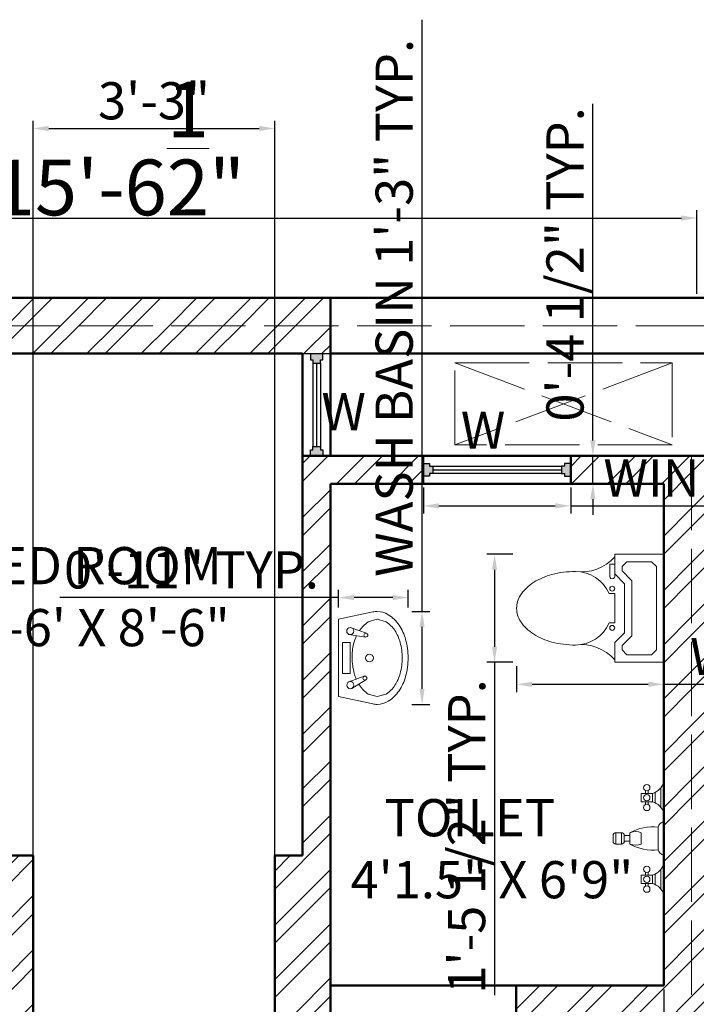
# Model space of a CAD drawing. Units: millimetres. Extents: x 4237 to 5109, y 21391 to 22486.
# Tile 9 of 17: x 4349 to 4458, y 22327 to 22486. Entities that reach past the tile are written whole.
import ezdxf

# ---------------------------------------------------------------- set-up
doc = ezdxf.new("R2010")
doc.units = ezdxf.units.MM
doc.linetypes.add('ACAD_ISO02W100', pattern=[15, 12, -3])
for name, color, linetype, lineweight in [('A-ANNO-DIMS', 2, 'Continuous', 18), ('A-ANNO-TEXT', 7, 'Continuous', 18), ('A-AREA-IDEN', 3, 'Continuous', 18), ('A-FLOR-OVHD', 1, 'ACAD_ISO02W100', 18), ('A-FURN', 8, 'Continuous', 18), ('A-WALL', 7, 'Continuous', 50), ('A-WALL-PATT', 252, 'Continuous', 13), ('windows', 140, 'Continuous', 25)]:
    doc.layers.add(name, color=color, linetype=linetype, lineweight=lineweight)
doc.styles.get("Standard").update_dxf_attribs({"font": 'arial.ttf'})
doc.dimstyles.new('ISO-25', dxfattribs={"dimtxt": 6, "dimasz": 2.5, "dimexe": 1.25, "dimexo": 0.625, "dimtad": 1, "dimdec": 1, "dimlunit": 4, "dimtxsty": 'Standard', "dimcen": 2.5, "dimadec": 0, "dimazin": 0, "dimtfac": 1, "dimtdec": 1, "dimtmove": 0, "dimatfit": 3, "dimfxl": 1, "dimarcsym": 0})

# ---------------------------------------------------------------- blocks, each defined once
blk = doc.blocks.new('A$C60F95712')
for p, q in [((0.05, 0.45), (0.003, 0.2283)), ((0.55, 0.45), (0.05, 0.45)), ((0.597, 0.2283), (0.55, 0.45)), ((0.1448, 0.3831), (0.1814, 0.2836)), ((0.4, 0.425), (0.2, 0.425)), ((0.2, 0.425), (0.2, 0.375)), ((0.4, 0.375), (0.4, 0.425)), ((0.1035, 0.3639), (0.1588, 0.2727)), ((0.2, 0.375), (0.4, 0.375)), ((0.4514, 0.3804), (0.4348, 0.2751)), ((0.4953, 0.3684), (0.459, 0.2688))]:
    blk.add_line(p, q)
for points in [[(0.1307, 0.319, 0.008163), (0.1232, 0.3143, 0.107176), (0.0669, 0.2578), (0.05, 0.2), (0.0669, 0.1422, 0.107176), (0.1232, 0.0857, 0.078233), (0.2003, 0.0515, 0.065516), (0.3, 0.0383, 0.065516), (0.3997, 0.0515, 0.078233), (0.4768, 0.0857, 0.107176), (0.5331, 0.1422), (0.55, 0.2)], [(0.4439, 0.3328, 0.046779), (0.3911, 0.3524, 0.080145), (0.3, 0.3617, 0.065516), (0.2003, 0.3485, 0.037125), (0.1623, 0.3353, 0.107176)], [(0.55, 0.2), (0.5331, 0.2578, 0.107176), (0.4768, 0.3143, 0.000976), (0.4758, 0.3149, 0.080145)]]:
    blk.add_lwpolyline(points, format="xyb")
for centre, radius in [((0.1241, 0.3735), 0.0228), ((0.4733, 0.3744), 0.0228), ((0.1696, 0.2793), 0.0126), ((0.3, 0.25), 0.025), ((0.4472, 0.2731), 0.0126)]:
    blk.add_circle(centre, radius)
for centre, radius, start, end in [((0.1362, 0.2), 0.1362, 168.02396, 180), ((0.1362, 0.2), 0.1362, 180, 211.85353), ((0.4638, 0.2), 0.1362, 328.14647, 0), ((0.4638, 0.2), 0.1362, 0, 11.97604), ((0.2147, 0.2488), 0.2286, 211.85353, 236.30993), ((0.3853, 0.2488), 0.2286, 303.69007, 328.14647), ((0.2662, 0.3261), 0.3215, 236.30993, 254.56292), ((0.3, 0.4484), 0.4484, 254.56292, 270), ((0.3, 0.4484), 0.4484, 270, 285.43708), ((0.3338, 0.3261), 0.3215, 285.43708, 303.69007)]:
    blk.add_arc(centre, radius, start, end)
blk = doc.blocks.new('A$C5EF6120A')
at = {"linetype": 'ByBlock'}
for p, q in [((0, 0.762), (0, 0.508)), ((0, 0.762), (0.5588, 0.762)), ((0.0381, 0.6985), (0.0635, 0.7239)), ((0.0635, 0.7239), (0.4953, 0.7239)), ((0.4953, 0.7239), (0.5207, 0.6985)), ((0.5588, 0.762), (0.5588, 0.508)), ((0.0381, 0.6985), (0.0381, 0.5715)), ((0.5207, 0.6985), (0.5207, 0.5715)), ((0.0635, 0.5461), (0.0381, 0.5715)), ((0.1366, 0.5969), (0.0858, 0.5461)), ((0.1366, 0.5969), (0.4222, 0.5969)), ((0.4222, 0.5969), (0.473, 0.5461)), ((0.5207, 0.5715), (0.4953, 0.5461)), ((0.0635, 0.5461), (0.0858, 0.5461)), ((0.1524, 0.5588), (0.1016, 0.508)), ((0.1524, 0.5588), (0.4064, 0.5588)), ((0.4064, 0.5588), (0.4572, 0.508)), ((0.4953, 0.5461), (0.473, 0.5461)), ((0, 0.508), (0.1016, 0.508)), ((0.0508, 0.508), (0.0508, 0.4826)), ((0.0508, 0.4826), (0.1143, 0.4826)), ((0.1143, 0.508), (0.1016, 0.508)), ((0.2032, 0.508), (0.2032, 0.4794)), ((0.3556, 0.508), (0.2032, 0.508)), ((0.3556, 0.508), (0.3556, 0.4794)), ((0.5588, 0.508), (0.4572, 0.508))]:
    blk.add_line(p, q, dxfattribs=at)
blk.add_lwpolyline([(0.0889, 0.3048, 0.063415), (0.1044, 0.183, 0.076468), (0.1447, 0.0893, 0.107136), (0.2118, 0.0204, 0.147373), (0.2794, 0, 0.147373), (0.347, 0.0204, 0.107136), (0.4141, 0.0893, 0.076468), (0.4544, 0.183, 0.063415), (0.4699, 0.3048, 0.063415)], format="xyb", dxfattribs=at)
for centre in [(0.1778, 0.4953), (0.381, 0.4953)]:
    blk.add_circle(centre, 0.0127, dxfattribs=at)
for centre, radius, start, end in [((-0.1375, 0.3358), 0.2285, 352.2011, 48.911), ((0.2794, 0.3048), 0.1905, 113.5782, 180), ((0.1143, 0.4953), 0.0127, 270, 90), ((0.2794, 0.3048), 0.1905, 0, 66.4218), ((0.6963, 0.3358), 0.2285, 131.089, 187.7989)]:
    blk.add_arc(centre, radius, start, end, dxfattribs=at)
blk = doc.blocks.new('Faucet - Bathroom front')
for p, q in [((-0.5, 4.25), (0.5, 4.25)), ((0.5, 3.75), (-0.5, 3.75)), ((-0.25, 3), (-0.25, 3.5)), ((0.25, 3.5), (0.25, 3)), ((-0.5, 3), (0.5, 3)), ((0.5, 2), (-0.5, 2)), ((-4, 1.625), (-4.25, 1.625)), ((-4, 1.375), (-4.25, 1.375)), ((-3.25, 1.625), (-3, 1.625)), ((-3.25, 1.375), (-3, 1.375)), ((3.25, 1.625), (3, 1.625)), ((3.25, 1.375), (3, 1.375)), ((4, 1.625), (4.25, 1.625)), ((4, 1.375), (4.25, 1.375)), ((-5, 0), (-2.25, 0)), ((-4.5087, 0.25), (-2.7408, 0.25)), ((-3.1442, 0.75), (-4.0979, 0.75)), ((-1.5, 0), (1.5, 0)), ((-1, 0.5), (1, 0.5)), ((2.25, 0), (5, 0)), ((2.7413, 0.25), (4.5092, 0.25)), ((4.1058, 0.75), (3.1521, 0.75))]:
    blk.add_line(p, q)
for points in [[(-0.25, 4.5), (0.25, 4.5)], [(-0.5, 3.75), (-0.5, 4.25)], [(0.25, 3.5), (-0.25, 3.5)], [(0.5, 4.25), (0.5, 3.75)]]:
    blk.add_lwpolyline(points)
for points in [[(-4, 1), (-4, 2), (-3.25, 2), (-3.25, 1)], [(3.25, 1), (3.25, 2), (4, 2), (4, 1)]]:
    blk.add_lwpolyline(points, close=True)
for centre in [(-4.5, 1.5), (-3.625, 1.5), (-2.75, 1.5), (2.75, 1.5), (3.625, 1.5), (4.5, 1.5)]:
    blk.add_circle(centre, 0.2795)
for centre, radius, start, end in [((-0.2575, 4.2575), 0.2426, 88.22243, 181.7776), ((0.2575, 4.2575), 0.2426, 358.2224, 91.77757), ((-0.2575, 3.7425), 0.2426, 178.2224, 271.7776), ((0.2575, 3.7425), 0.2426, 268.2224, 1.777565), ((3, 1), 4.0311, 150.2551, 187.125), ((0.6413, 2.5), 1.246, 156.3417, 203.6583), ((-3, 1), 4.0311, 352.875, 29.74488), ((-0.6413, 2.5), 1.246, 336.3417, 23.65835), ((-5.375, 1.375), 1.4252, 285.2551, 344.7449), ((-1.875, 1.375), 1.4252, 195.2551, 254.7449), ((1.875, 1.375), 1.4252, 285.2551, 344.7449), ((5.375, 1.375), 1.4252, 195.2551, 254.7449), ((-0.7962, -0.2038), 0.7327, 106.1502, 163.8498), ((0.7962, -0.2038), 0.7327, 16.1502, 73.84979)]:
    blk.add_arc(centre, radius, start, end)
blk = doc.blocks.new('*D56')
at = {"layer": 'A-ANNO-DIMS', "color": 0, "lineweight": -2, "transparency": 16777216}
for p, q in [((4271.65, 22441.33), (4271.65, 22454.84)), ((4458.3, 22441.33), (4458.3, 22454.84)), ((4274.15, 22453.59), (4455.8, 22453.59))]:
    blk.add_line(p, q, dxfattribs=at)
at = {"layer": 'A-ANNO-DIMS', "color": 0, "transparency": 16777216}
for points in [[(4274.15, 22454.01), (4274.15, 22453.17), (4271.65, 22453.59)], [(4455.8, 22454.01), (4455.8, 22453.17), (4458.3, 22453.59)]]:
    blk.add_solid(points, dxfattribs=at)
at = {"layer": 'Defpoints', "color": 0, "transparency": 16777216}
for p in [(4458.3, 22453.59), (4271.65, 22440.7), (4458.3, 22440.7)]:
    blk.add_point(p, dxfattribs=at)
at = {"layer": 'A-ANNO-DIMS', "color": 0, "transparency": 16777216, "insert": (4364.98, 22464.83), "char_height": 9, "attachment_point": 5}
blk.add_mtext('15\'-6{\\H1x;\\S1/2;}"', dxfattribs=at)
blk = doc.blocks.new('WIN-A')
blk.add_line((0, 4.5), (0, 0))
blk.add_lwpolyline([(0, 4.5), (23.8, 4.5), (23.8, 0), (0, 0)], close=True)
blk = doc.blocks.new('*D74')
at = {"layer": 'A-ANNO-DIMS', "color": 0, "lineweight": -2, "transparency": 16777216}
for p, q in [((4413.94, 22390.08), (4413.94, 22485.61)), ((4412.31, 22390.08), (4415.19, 22390.08)), ((4413.94, 22377.59), (4413.94, 22387.58)), ((4412.31, 22375.09), (4415.19, 22375.09))]:
    blk.add_line(p, q, dxfattribs=at)
at = {"layer": 'A-ANNO-DIMS', "color": 0, "transparency": 16777216}
for points in [[(4413.52, 22387.58), (4414.35, 22387.58), (4413.94, 22390.08)], [(4413.52, 22377.59), (4414.35, 22377.59), (4413.94, 22375.09)]]:
    blk.add_solid(points, dxfattribs=at)
at = {"layer": 'Defpoints', "color": 0, "transparency": 16777216}
for p in [(4411.69, 22390.08), (4413.94, 22390.08), (4411.69, 22375.09)]:
    blk.add_point(p, dxfattribs=at)
at = {"layer": 'A-ANNO-DIMS', "color": 0, "transparency": 16777216, "insert": (4410.21, 22439.09), "char_height": 6, "attachment_point": 5, "rotation": 90}
blk.add_mtext('WASH BASIN 1\'-3" TYP.', dxfattribs=at)
blk = doc.blocks.new('*D75')
at = {"layer": 'A-ANNO-DIMS', "color": 0, "lineweight": -2, "transparency": 16777216}
for p, q in [((4400.45, 22390.71), (4400.45, 22393.58)), ((4411.69, 22390.71), (4411.69, 22393.58)), ((4400.45, 22392.33), (4355.46, 22392.33)), ((4409.19, 22392.33), (4402.95, 22392.33))]:
    blk.add_line(p, q, dxfattribs=at)
at = {"layer": 'A-ANNO-DIMS', "color": 0, "transparency": 16777216}
for points in [[(4402.95, 22392.75), (4402.95, 22391.91), (4400.45, 22392.33)], [(4409.19, 22392.75), (4409.19, 22391.91), (4411.69, 22392.33)]]:
    blk.add_solid(points, dxfattribs=at)
at = {"layer": 'Defpoints', "color": 0, "transparency": 16777216}
for p in [(4400.45, 22392.33), (4400.45, 22390.08), (4411.69, 22390.08)]:
    blk.add_point(p, dxfattribs=at)
at = {"layer": 'A-ANNO-DIMS', "color": 0, "transparency": 16777216, "insert": (4376.7, 22396.02), "char_height": 6, "attachment_point": 5}
blk.add_mtext('0\'-11" TYP.', dxfattribs=at)
blk = doc.blocks.new('*D76')
at = {"layer": 'A-ANNO-DIMS', "color": 0, "lineweight": -2, "transparency": 16777216}
for p, q in [((4429.2, 22381.26), (4429.2, 22377.08)), ((4452.95, 22381.26), (4452.95, 22377.08)), ((4431.7, 22378.33), (4450.45, 22378.33)), ((4452.95, 22378.33), (4509.81, 22378.33))]:
    blk.add_line(p, q, dxfattribs=at)
at = {"layer": 'A-ANNO-DIMS', "color": 0, "transparency": 16777216}
for points in [[(4431.7, 22378.74), (4431.7, 22377.91), (4429.2, 22378.33)], [(4450.45, 22378.74), (4450.45, 22377.91), (4452.95, 22378.33)]]:
    blk.add_solid(points, dxfattribs=at)
at = {"layer": 'Defpoints', "color": 0, "transparency": 16777216}
for p in [(4429.2, 22381.89), (4452.95, 22381.89), (4452.95, 22378.33)]:
    blk.add_point(p, dxfattribs=at)
at = {"layer": 'A-ANNO-DIMS', "color": 0, "transparency": 16777216, "insert": (4482.63, 22382.05), "char_height": 6, "attachment_point": 5}
blk.add_mtext('WC 2\'-0" TYP.', dxfattribs=at)
blk = doc.blocks.new('*D77')
at = {"layer": 'A-ANNO-DIMS', "color": 0, "lineweight": -2, "transparency": 16777216}
for p, q in [((4428.57, 22399.31), (4424.39, 22399.31)), ((4425.64, 22396.81), (4425.64, 22384.39)), ((4428.57, 22381.89), (4424.39, 22381.89)), ((4425.64, 22381.89), (4425.64, 22328.15))]:
    blk.add_line(p, q, dxfattribs=at)
at = {"layer": 'A-ANNO-DIMS', "color": 0, "transparency": 16777216}
for points in [[(4425.22, 22396.81), (4426.05, 22396.81), (4425.64, 22399.31)], [(4425.22, 22384.39), (4426.05, 22384.39), (4425.64, 22381.89)]]:
    blk.add_solid(points, dxfattribs=at)
at = {"layer": 'Defpoints', "color": 0, "transparency": 16777216}
for p in [(4429.2, 22399.31), (4425.64, 22381.89), (4429.2, 22381.89)]:
    blk.add_point(p, dxfattribs=at)
at = {"layer": 'A-ANNO-DIMS', "color": 0, "transparency": 16777216, "insert": (4421.91, 22353.77), "char_height": 6, "attachment_point": 5, "rotation": 90}
blk.add_mtext('1\'-5 1/2" TYP.', dxfattribs=at)
blk = doc.blocks.new('*D80')
at = {"layer": 'A-ANNO-DIMS', "color": 0, "lineweight": -2, "transparency": 16777216}
for p, q in [((4414.15, 22410.08), (4414.15, 22405.88)), ((4437.95, 22410.08), (4437.95, 22405.88)), ((4416.65, 22407.13), (4435.45, 22407.13)), ((4437.95, 22407.13), (4527.87, 22407.13))]:
    blk.add_line(p, q, dxfattribs=at)
at = {"layer": 'A-ANNO-DIMS', "color": 0, "transparency": 16777216}
for points in [[(4416.65, 22407.55), (4416.65, 22406.71), (4414.15, 22407.13)], [(4435.45, 22407.55), (4435.45, 22406.71), (4437.95, 22407.13)]]:
    blk.add_solid(points, dxfattribs=at)
at = {"layer": 'Defpoints', "color": 0, "transparency": 16777216}
for p in [(4414.15, 22410.7), (4437.95, 22410.7), (4437.95, 22407.13)]:
    blk.add_point(p, dxfattribs=at)
at = {"layer": 'A-ANNO-DIMS', "color": 0, "transparency": 16777216, "insert": (4484.16, 22410.86), "char_height": 6, "attachment_point": 5}
blk.add_mtext('WINDOW W 2\'-0" TYP.', dxfattribs=at)
blk = doc.blocks.new('*D81')
at = {"layer": 'A-ANNO-DIMS', "color": 0, "lineweight": -2, "transparency": 16777216}
for p, q in [((4441.52, 22417.7), (4441.52, 22472)), ((4438.58, 22415.2), (4442.77, 22415.2)), ((4441.52, 22410.7), (4441.52, 22415.2)), ((4438.58, 22410.7), (4442.77, 22410.7)), ((4441.52, 22408.2), (4441.52, 22405.7))]:
    blk.add_line(p, q, dxfattribs=at)
at = {"layer": 'A-ANNO-DIMS', "color": 0, "transparency": 16777216}
for points in [[(4441.1, 22417.7), (4441.94, 22417.7), (4441.52, 22415.2)], [(4441.1, 22408.2), (4441.94, 22408.2), (4441.52, 22410.7)]]:
    blk.add_solid(points, dxfattribs=at)
at = {"layer": 'Defpoints', "color": 0, "transparency": 16777216}
for p in [(4437.95, 22415.2), (4441.52, 22415.2), (4437.95, 22410.7)]:
    blk.add_point(p, dxfattribs=at)
at = {"layer": 'A-ANNO-DIMS', "color": 0, "transparency": 16777216, "insert": (4437.79, 22446.1), "char_height": 6, "attachment_point": 5, "rotation": 90}
blk.add_mtext('0\'-4 1/2" TYP.', dxfattribs=at)
blk = doc.blocks.new('*D109')
at = {"layer": 'A-ANNO-DIMS', "color": 0, "lineweight": -2, "transparency": 16777216}
for p, q in [((4351.15, 22325.83), (4351.15, 22469.3)), ((4390.15, 22325.83), (4390.15, 22469.3)), ((4353.65, 22468.05), (4387.65, 22468.05))]:
    blk.add_line(p, q, dxfattribs=at)
at = {"layer": 'A-ANNO-DIMS', "color": 0, "transparency": 16777216}
for points in [[(4353.65, 22468.47), (4353.65, 22467.63), (4351.15, 22468.05)], [(4387.65, 22468.47), (4387.65, 22467.63), (4390.15, 22468.05)]]:
    blk.add_solid(points, dxfattribs=at)
at = {"layer": 'Defpoints', "color": 0, "transparency": 16777216}
for p in [(4390.15, 22468.05), (4351.15, 22325.2), (4390.15, 22325.2)]:
    blk.add_point(p, dxfattribs=at)
at = {"layer": 'A-ANNO-DIMS', "color": 0, "transparency": 16777216, "insert": (4370.65, 22471.74), "char_height": 6, "attachment_point": 5}
blk.add_mtext('3\'-3"', dxfattribs=at)
blk = doc.blocks.new('*D110')
at = {"layer": 'A-ANNO-DIMS', "color": 0, "lineweight": -2, "transparency": 16777216}
for p, q in [((4399.15, 22329.08), (4399.15, 21960.6)), ((4452.95, 22329.08), (4452.95, 21960.6)), ((4401.65, 21961.85), (4450.45, 21961.85))]:
    blk.add_line(p, q, dxfattribs=at)
at = {"layer": 'A-ANNO-DIMS', "color": 0, "transparency": 16777216}
for points in [[(4401.65, 21962.27), (4401.65, 21961.43), (4399.15, 21961.85)], [(4450.45, 21962.27), (4450.45, 21961.43), (4452.95, 21961.85)]]:
    blk.add_solid(points, dxfattribs=at)
at = {"layer": 'Defpoints', "color": 0, "transparency": 16777216}
for p in [(4399.15, 22329.7), (4452.95, 22329.7), (4452.95, 21961.85)]:
    blk.add_point(p, dxfattribs=at)
at = {"layer": 'A-ANNO-DIMS', "color": 0, "transparency": 16777216, "insert": (4426.05, 21965.54), "char_height": 6, "attachment_point": 5}
blk.add_mtext('4\'-6"', dxfattribs=at)

msp = doc.modelspace()

# ---------------------------------------------------------------- hatches: boundary and pattern name
at = {"layer": 'A-WALL-PATT'}
h = msp.add_hatch(dxfattribs=at)
h.set_pattern_fill('ANSI32', color=256, scale=0.65)
h.paths.add_polyline_path([(4399.15, 22440.7), (4271.65, 22440.7), (4271.65, 22032.7), (4276.15, 22032.7), (4276.15, 22044.7), (4276.15, 22436.2), (4399.15, 22436.2)])
h.paths.add_polyline_path([(4351.15, 22185.7), (4357.15, 22185.7), (4357.15, 22194.7), (4346.65, 22194.7), (4346.65, 22080.7), (4351.15, 22080.7)], flags=16)
h.paths.add_polyline_path([(4351.15, 22295.2), (4346.65, 22295.2), (4346.65, 22238.2), (4311.53, 22238.2), (4311.53, 22233.7), (4351.15, 22233.7)], flags=16)
h = msp.add_hatch(dxfattribs=at)
h.set_pattern_fill('ANSI32', color=256, scale=0.65)
h.paths.add_polyline_path([(4399.15, 22436.2), (4276.15, 22436.2), (4276.15, 22044.7), (4280.65, 22044.7), (4280.65, 22233.7), (4287.73, 22233.7), (4287.73, 22238.2), (4280.65, 22238.2), (4280.65, 22325.2), (4351.15, 22325.2), (4351.15, 22350.7), (4346.65, 22350.7), (4346.65, 22329.7), (4280.65, 22329.7), (4280.65, 22431.7), (4394.65, 22431.7), (4399.15, 22431.7)], flags=17)
h.paths.add_polyline_path([(4351.15, 22185.7), (4357.15, 22185.7), (4357.15, 22194.7), (4346.65, 22194.7), (4346.65, 22080.7), (4351.15, 22080.7)], flags=16)
h.paths.add_polyline_path([(4351.15, 22295.2), (4346.65, 22295.2), (4346.65, 22238.2), (4311.53, 22238.2), (4311.53, 22233.7), (4351.15, 22233.7)], flags=16)
h = msp.add_hatch(color=256, dxfattribs=at)
h.dxf.hatch_style = 1
h.paths.add_polyline_path([(4397.51, 22430.7), (4397.9, 22430.7), (4397.9, 22431.7), (4395.9, 22431.7), (4395.9, 22430.7), (4396.29, 22430.7), (4396.29, 22430.19), (4397.51, 22430.19)])
h = msp.add_hatch(color=256, dxfattribs=at)
h.dxf.hatch_style = 1
h.paths.add_polyline_path([(4397.9, 22416.2), (4397.51, 22416.2), (4397.51, 22416.71), (4396.29, 22416.71), (4396.29, 22416.2), (4395.9, 22416.2), (4395.9, 22415.2), (4397.9, 22415.2)])
h = msp.add_hatch(dxfattribs=at)
h.set_pattern_fill('ANSI32', color=256, scale=0.65)
h.paths.add_polyline_path([(4399.15, 22410.7), (4414.15, 22410.7), (4414.15, 22415.2), (4394.65, 22415.2), (4394.65, 22350.7), (4390.15, 22350.7), (4390.15, 22325.2), (4399.15, 22325.2)])
h = msp.add_hatch(dxfattribs=at)
h.set_pattern_fill('ANSI32', color=256, scale=0.65)
h.paths.add_polyline_path([(4457.45, 22415.2), (4437.95, 22415.2), (4437.95, 22410.7), (4452.95, 22410.7), (4452.95, 22329.7), (4429.15, 22329.7), (4429.15, 22325.2), (4452.95, 22325.2), (4452.95, 22233.7), (4457.45, 22233.7)])
h = msp.add_hatch(dxfattribs=at)
h.set_pattern_fill('ANSI32', color=256, scale=0.65)
h.paths.add_polyline_path([(4461.95, 22415.2), (4457.45, 22415.2), (4457.45, 22233.7), (4461.95, 22233.7)])
h = msp.add_hatch(color=256, dxfattribs=at)
h.dxf.hatch_style = 1
h.paths.add_polyline_path([(4415.67, 22413.56), (4415.15, 22413.56), (4415.15, 22413.95), (4414.15, 22413.95), (4414.15, 22411.95), (4415.15, 22411.95), (4415.15, 22412.34), (4415.67, 22412.34)])
h = msp.add_hatch(color=256, dxfattribs=at)
h.dxf.hatch_style = 1
h.paths.add_polyline_path([(4437.95, 22413.95), (4436.95, 22413.95), (4436.95, 22413.56), (4436.44, 22413.56), (4436.44, 22412.34), (4436.95, 22412.34), (4436.95, 22411.95), (4437.95, 22411.95)])

# ---------------------------------------------------------------- linework, layer by layer
at = {"layer": 'A-FLOR-OVHD'}
for p, q in [((4419.22, 22430.2), (4454.33, 22416.99)), ((4454.33, 22430.2), (4419.22, 22416.99)), ((4457.45, 22415.2), (4457.45, 22032.7))]:
    msp.add_line(p, q, dxfattribs=at)
msp.add_lwpolyline([(4640.45, 22032.7), (4640.45, 22436.2), (4276.15, 22436.2), (4276.15, 22032.7)], dxfattribs=at)
msp.add_lwpolyline([(4419.22, 22430.2), (4454.33, 22430.2), (4454.33, 22416.99), (4419.22, 22416.99)], close=True, dxfattribs=at)
at = {"layer": 'A-WALL'}
for p, q in [((4271.65, 22440.7), (4644.95, 22440.7)), ((4399.15, 22440.7), (4399.15, 22415.2)), ((4280.65, 22431.7), (4394.65, 22431.7)), ((4394.65, 22431.7), (4394.65, 22350.7)), ((4399.15, 22431.7), (4517.45, 22431.7)), ((4394.65, 22415.2), (4521.95, 22415.2)), ((4437.95, 22415.2), (4437.95, 22410.7)), ((4399.15, 22410.7), (4452.95, 22410.7)), ((4399.15, 22410.7), (4399.15, 22325.2)), ((4452.95, 22410.7), (4452.95, 22329.7)), ((4280.65, 22350.7), (4351.15, 22350.7)), ((4351.15, 22350.7), (4351.15, 22325.2)), ((4390.15, 22350.7), (4390.15, 22325.2)), ((4390.15, 22350.7), (4394.65, 22350.7)), ((4429.15, 22329.7), (4399.15, 22329.7)), ((4429.15, 22329.7), (4452.95, 22329.7)), ((4429.15, 22329.7), (4429.15, 22325.2))]:
    msp.add_line(p, q, dxfattribs=at)
at = {"layer": 'windows'}
for p, q in [((4396.29, 22430.19), (4396.29, 22416.71)), ((4396.9, 22430.19), (4396.9, 22416.71)), ((4397.51, 22430.19), (4397.51, 22416.71)), ((4415.67, 22413.56), (4436.44, 22413.56)), ((4415.67, 22412.95), (4436.44, 22412.95)), ((4436.44, 22412.34), (4415.67, 22412.34))]:
    msp.add_line(p, q, dxfattribs=at)
msp.add_lwpolyline([(4394.65, 22431.7), (4399.15, 22431.7), (4399.15, 22415.2), (4394.65, 22415.2)], close=True, dxfattribs=at)
for points in [[(4395.9, 22431.7), (4395.9, 22430.7), (4396.29, 22430.7), (4396.29, 22430.19), (4397.51, 22430.19), (4397.51, 22430.7), (4397.9, 22430.7), (4397.9, 22431.7)], [(4395.9, 22415.2), (4395.9, 22416.2), (4396.29, 22416.2), (4396.29, 22416.71), (4397.51, 22416.71), (4397.51, 22416.2), (4397.9, 22416.2), (4397.9, 22415.2)], [(4414.15, 22413.95), (4415.15, 22413.95), (4415.15, 22413.56), (4415.67, 22413.56), (4415.67, 22412.34), (4415.15, 22412.34), (4415.15, 22411.95), (4414.15, 22411.95)], [(4437.95, 22413.95), (4436.95, 22413.95), (4436.95, 22413.56), (4436.44, 22413.56), (4436.44, 22412.34), (4436.95, 22412.34), (4436.95, 22411.95), (4437.95, 22411.95)]]:
    msp.add_lwpolyline(points, dxfattribs=at)

# ---------------------------------------------------------------- block references
at = {"layer": 'A-FURN'}
for name, p, xscale, yscale, zscale, rotation in [('A$C5EF6120A', (4429.2, 22399.31), 31.17096342775826, 31.17096342775826, 31.17096342775826, 270), ('A$C60F95712', (4411.69, 22375.09), 24.98450815685876, 24.98450815685876, 24.98450815685876, 90), ('Faucet - Bathroom front', (4452.95, 22353.45), 1.818895909746216, 1.818895909746216, 1.818895909746216, 90)]:
    msp.add_blockref(name, p, dxfattribs=dict(at, xscale=xscale, yscale=yscale, zscale=zscale, rotation=rotation))
at = {"layer": 'windows'}
msp.add_blockref('WIN-A', (4414.15, 22410.7), dxfattribs=at)

# ---------------------------------------------------------------- texts
at = {"layer": 'A-ANNO-TEXT', "char_height": 6, "attachment_point": 1}
for insert in [(4390.35, 22425.35), (4412.86, 22422.35)]:
    msp.add_mtext_dynamic_manual_height_columns('    W', width=21.7253, gutter_width=12.5, heights=[0], dxfattribs=dict(at, insert=insert))
at = {"layer": 'A-AREA-IDEN', "char_height": 6, "attachment_point": 1}
for s, insert in [('BED ROOM \\P9\'-6\' X 8\'-6"', (4339.96, 22400.48)), ('   TOILET\\P4\'1.5" X 6\'9"', (4402.38, 22359.79))]:
    msp.add_mtext_dynamic_manual_height_columns(s, width=55.7646, gutter_width=12.5, heights=[0], dxfattribs=dict(at, insert=insert))

# ---------------------------------------------------------------- dimensions: what is measured, and where the dimension line sits
at = {"layer": 'A-ANNO-DIMS'}
for base, p1, p2, angle, text, picture, middle in [((4413.94, 22390.08), (4411.69, 22375.09), (4411.69, 22390.08), 90, 'WASH BASIN <> TYP.', '*D74', (4410.21, 22439.09)), ((4441.52, 22415.2), (4437.95, 22410.7), (4437.95, 22415.2), 90, '<> TYP.', '*D81', (4437.79, 22446.1)), ((4400.45, 22392.33), (4411.69, 22390.08), (4400.45, 22390.08), 180, '<> TYP.', '*D75', (4376.7, 22396.02)), ((4425.64, 22381.89), (4429.2, 22399.31), (4429.2, 22381.89), 270, '<> TYP.', '*D77', (4421.91, 22353.77))]:
    dim = msp.add_linear_dim(base=base, p1=p1, p2=p2, angle=angle, text=text, dimstyle='ISO-25', override={"dimdec": 1, "dimrnd": 0, "dimzin": 1, "dimlunit": 4, "dimfrac": 2}, dxfattribs=at)
    dim.commit()
    dim.dimension.update_dxf_attribs({"geometry": picture, "text_midpoint": middle})
for base, p1, p2, override, picture, middle in [((4458.30138825, 22453.59015802), (4271.65138825, 22440.70062861), (4458.30138825, 22440.70062861), {"dimtxt": 9, "dimclrd": 0, "dimclre": 0, "dimclrt": 0}, '*D56', (4364.97638825, 22464.82873237)), ((4390.15, 22468.05), (4351.15, 22325.2), (4390.15, 22325.2), {"dimdec": 1, "dimlfac": 1, "dimrnd": 0, "dimzin": 1, "dimdsep": 46, "dimlunit": 4, "dimfrac": 2}, '*D109', (4370.65, 22471.74)), ((4452.95, 21961.85), (4399.15, 22329.7), (4452.95, 22329.7), {"dimdec": 1, "dimlfac": 1, "dimrnd": 0, "dimzin": 1, "dimdsep": 46, "dimlunit": 4, "dimfrac": 2}, '*D110', (4426.05, 21965.54))]:
    dim = msp.add_linear_dim(base=base, p1=p1, p2=p2, dimstyle='ISO-25', override=override, dxfattribs=at)
    dim.commit()
    dim.dimension.update_dxf_attribs({"geometry": picture, "text_midpoint": middle})
for base, p1, p2, text, picture, middle in [((4437.95, 22407.13), (4414.15, 22410.7), (4437.95, 22410.7), 'WINDOW W <> TYP.', '*D80', (4484.16, 22410.86)), ((4452.9514, 22378.3263), (4429.1991, 22381.8892), (4452.9514, 22381.8892), 'WC <> TYP.', '*D76', (4482.6323, 22382.0536))]:
    dim = msp.add_linear_dim(base=base, p1=p1, p2=p2, text=text, dimstyle='ISO-25', override={"dimdec": 1, "dimrnd": 0, "dimzin": 1, "dimlunit": 4, "dimfrac": 2}, dxfattribs=at)
    dim.commit()
    dim.dimension.update_dxf_attribs({"geometry": picture, "text_midpoint": middle})

doc.saveas('drawing.dxf')
